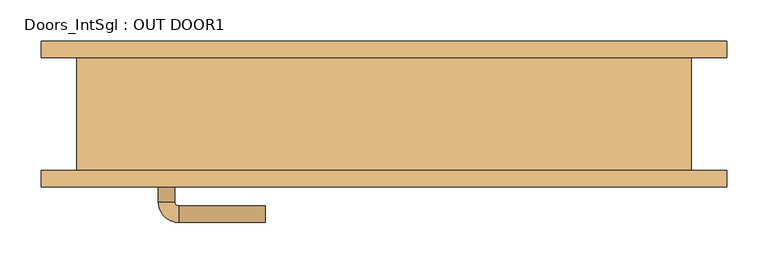
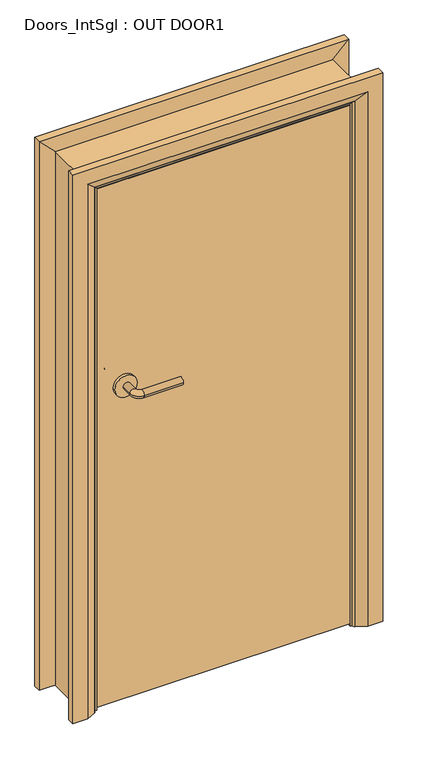
"""IFC4 building model written with IfcOpenShell, lengths in millimetres: door geometry, Doors_IntSgl : OUT DOOR1."""

from ifc_helpers import new_model, si_unit, point, frame, frame_2d, origin, place, context, project, spatial, polyline, circle_curve, ellipse_curve, trimmed, segment, composite_curve, outline, extrude, faceted_brep, source, transform, mapped, element, save
from ifc_brep_helpers import plane_surface, cylinder_surface, revolved_surface, advanced_brep


def doors_intsgl_out_door1_d16f2837(model_context):
    return source(origin(), model_context, "Body", "SolidModel", [
        advanced_brep(
        [(-274.0, -22.58, 900.0), (-254.0, -22.58, 900.0), (-274.0, 7.42, 900.0), (-254.0, 7.42, 900.0), (-249.0, 12.42, 900.0), (-249.0, 32.42, 900.0), (-144.0, 32.42, 900.0), (-144.0, 12.42, 900.0)],
        [
            (0, 1, circle_curve(frame((-264.0, -22.58, 900.0), z_axis=(0.0, -1.0, 0.0), x_axis=(1.0, 0.0, 0.0)), 10.0)),
            (1, 0, circle_curve(frame((-264.0, -22.58, 900.0), z_axis=(0.0, -1.0, 0.0), x_axis=(1.0, 0.0, 0.0)), 10.0)),
            (0, 2),
            (2, 3, circle_curve(frame((-264.0, 7.42, 900.0), z_axis=(0.0, -1.0, 0.0), x_axis=(1.0, 0.0, 0.0)), 10.0)),
            (3, 1),
            (3, 2, circle_curve(frame((-264.0, 7.42, 900.0), z_axis=(0.0, -1.0, 0.0), x_axis=(1.0, 0.0, 0.0)), 10.0)),
            (4, 3, circle_curve(frame((-249.0, 7.42, 900.0), z_axis=(0.0, 0.0, 1.0), x_axis=(-1.0, 0.0, 0.0)), 5.0)),
            (2, 5, circle_curve(frame((-249.0, 7.42, 900.0), z_axis=(0.0, 0.0, -1.0), x_axis=(-1.0, 0.0, 0.0)), 25.0)),
            (5, 4, circle_curve(frame((-249.0, 22.42, 900.0), z_axis=(-1.0, 0.0, 0.0), x_axis=(0.0, -1.0, 0.0)), 10.0)),
            (4, 5, circle_curve(frame((-249.0, 22.42, 900.0), z_axis=(-1.0, 0.0, 0.0), x_axis=(0.0, -1.0, 0.0)), 10.0)),
            (6, 7, circle_curve(frame((-144.0, 22.42, 900.0), z_axis=(1.0, 0.0, 0.0), x_axis=(0.0, -1.0, 0.0)), 10.0)),
            (7, 6, circle_curve(frame((-144.0, 22.42, 900.0), z_axis=(1.0, 0.0, 0.0), x_axis=(0.0, -1.0, 0.0)), 10.0)),
            (5, 6),
            (7, 4),
        ],
        [
            plane_surface(frame((-264.0, -22.58, 900.0), z_axis=(0.0, -1.0, 0.0), x_axis=(0.0, 0.0, 1.0))),
            cylinder_surface(frame((-264.0, -22.58, 900.0), z_axis=(0.0, -1.0, 0.0), x_axis=(1.0, 0.0, 0.0)), 10.0),
            revolved_surface(trimmed(ellipse_curve(frame((-264.0, 7.42, 900.0), z_axis=(0.0, -1.0, 0.0), x_axis=(1.0, 0.0, 0.0)), 10.0, 10.0), [point((-274.0, 7.42, 900.0))], [point((-254.0, 7.42, 900.0))], True, "CARTESIAN"), (-249.0, 7.42, 900.0), (0.0, 0.0, -1.0)),
            revolved_surface(trimmed(ellipse_curve(frame((-264.0, 7.42, 900.0), z_axis=(0.0, -1.0, 0.0), x_axis=(1.0, 0.0, 0.0)), 10.0, 10.0), [point((-254.0, 7.42, 900.0))], [point((-274.0, 7.42, 900.0))], True, "CARTESIAN"), (-249.0, 7.42, 900.0), (0.0, 0.0, -1.0)),
            plane_surface(frame((-144.0, 22.42, 900.0), z_axis=(1.0, 0.0, 0.0), x_axis=(0.0, 0.0, 1.0))),
            cylinder_surface(frame((-249.0, 22.42, 900.0), z_axis=(-1.0, 0.0, 0.0), x_axis=(0.0, -1.0, 0.0)), 10.0),
        ],
        [
            (0, [[1, 2]]),
            (1, [[-1, 3, 4, 5]]),
            (1, [[-2, -5, 6, -3]]),
            (2, [[7, -4, 8, 9]]),
            (3, [[-8, -6, -7, 10]]),
            (4, [[11, 12]]),
            (5, [[-9, 13, -12, 14]]),
            (5, [[-10, -14, -11, -13]]),
        ],
    ),
        extrude(outline(composite_curve([segment(trimmed(circle_curve(frame_2d((900.0, -266.5)), 30.0), [point((900.0, -296.5))], [point((900.0, -236.5))], False, "CARTESIAN"), True, "CONTINUOUS"), segment(trimmed(circle_curve(frame_2d((900.0, -266.5)), 30.0), [point((900.0, -236.5))], [point((900.0, -296.5))], False, "CARTESIAN"), True, "CONTINUOUS")], self_intersect=False)), frame((0.0, -30.58, 0.0), z_axis=(0.0, 1.0, 0.0), x_axis=(0.0, 0.0, 1.0)), (0.0, 0.0, 1.0), 8.0),
        advanced_brep(
        [(-274.0, -76.58, 900.0), (-254.0, -76.58, 900.0), (-254.0, -106.58, 900.0), (-274.0, -106.58, 900.0), (-249.0, -111.58, 900.0), (-249.0, -131.58, 900.0), (-144.0, -131.58, 900.0), (-144.0, -111.58, 900.0)],
        [
            (0, 1, circle_curve(frame((-264.0, -76.58, 900.0), z_axis=(0.0, 1.0, 0.0), x_axis=(1.0, 0.0, 0.0)), 10.0)),
            (1, 0, circle_curve(frame((-264.0, -76.58, 900.0), z_axis=(0.0, 1.0, 0.0), x_axis=(1.0, 0.0, 0.0)), 10.0)),
            (1, 2),
            (2, 3, circle_curve(frame((-264.0, -106.58, 900.0), z_axis=(0.0, 1.0, 0.0), x_axis=(1.0, 0.0, 0.0)), 10.0)),
            (3, 0),
            (3, 2, circle_curve(frame((-264.0, -106.58, 900.0), z_axis=(0.0, 1.0, 0.0), x_axis=(1.0, 0.0, 0.0)), 10.0)),
            (4, 5, circle_curve(frame((-249.0, -121.58, 900.0), z_axis=(-1.0, 0.0, 0.0), x_axis=(0.0, 1.0, 0.0)), 10.0)),
            (5, 3, circle_curve(frame((-249.0, -106.58, 900.0), z_axis=(0.0, 0.0, -1.0), x_axis=(-1.0, 0.0, 0.0)), 25.0)),
            (2, 4, circle_curve(frame((-249.0, -106.58, 900.0), z_axis=(0.0, 0.0, 1.0), x_axis=(-1.0, 0.0, 0.0)), 5.0)),
            (5, 4, circle_curve(frame((-249.0, -121.58, 900.0), z_axis=(-1.0, 0.0, 0.0), x_axis=(0.0, 1.0, 0.0)), 10.0)),
            (6, 7, circle_curve(frame((-144.0, -121.58, 900.0), z_axis=(1.0, 0.0, 0.0), x_axis=(0.0, 1.0, 0.0)), 10.0)),
            (7, 6, circle_curve(frame((-144.0, -121.58, 900.0), z_axis=(1.0, 0.0, 0.0), x_axis=(0.0, 1.0, 0.0)), 10.0)),
            (4, 7),
            (6, 5),
        ],
        [
            plane_surface(frame((-264.0, -76.58, 900.0), z_axis=(0.0, 1.0, 0.0), x_axis=(0.0, 0.0, 1.0))),
            cylinder_surface(frame((-264.0, -76.58, 900.0), z_axis=(0.0, 1.0, 0.0), x_axis=(1.0, 0.0, 0.0)), 10.0),
            revolved_surface(trimmed(ellipse_curve(frame((-264.0, -106.58, 900.0), z_axis=(0.0, -1.0, 0.0), x_axis=(1.0, 0.0, 0.0)), 10.0, 10.0), [point((-274.0, -106.58, 900.0))], [point((-254.0, -106.58, 900.0))], True, "CARTESIAN"), (-249.0, -106.58, 900.0), (0.0, 0.0, -1.0)),
            revolved_surface(trimmed(ellipse_curve(frame((-264.0, -106.58, 900.0), z_axis=(0.0, -1.0, 0.0), x_axis=(1.0, 0.0, 0.0)), 10.0, 10.0), [point((-254.0, -106.58, 900.0))], [point((-274.0, -106.58, 900.0))], True, "CARTESIAN"), (-249.0, -106.58, 900.0), (0.0, 0.0, -1.0)),
            plane_surface(frame((-144.0, -121.58, 900.0), z_axis=(1.0, 0.0, 0.0), x_axis=(0.0, 0.0, 1.0))),
            cylinder_surface(frame((-249.0, -121.58, 900.0), z_axis=(-1.0, 0.0, 0.0), x_axis=(0.0, 1.0, 0.0)), 10.0),
        ],
        [
            (0, [[1, 2]]),
            (1, [[3, 4, 5, -2]]),
            (1, [[-5, 6, -3, -1]]),
            (2, [[7, 8, -4, 9]]),
            (3, [[10, -9, -6, -8]]),
            (4, [[11, 12]]),
            (5, [[13, -11, 14, -7]]),
            (5, [[-14, -12, -13, -10]]),
        ],
    ),
        extrude(outline(composite_curve([segment(trimmed(circle_curve(frame_2d((900.0, -266.5)), 30.0), [point((900.0, -296.5))], [point((900.0, -236.5))], False, "CARTESIAN"), True, "CONTINUOUS"), segment(trimmed(circle_curve(frame_2d((900.0, -266.5)), 30.0), [point((900.0, -236.5))], [point((900.0, -296.5))], False, "CARTESIAN"), True, "CONTINUOUS")], self_intersect=False)), frame((0.0, -76.58, 0.0), z_axis=(0.0, 1.0, 0.0), x_axis=(0.0, 0.0, 1.0)), (0.0, 0.0, 1.0), 8.0),
        extrude(outline(polyline([(339.0, -30.58), (339.0, -68.58), (-339.0, -68.58), (-339.0, -30.58), (339.0, -30.58)])), frame((0.0, 0.0, 8.0), z_axis=(0.0, 0.0, 1.0), x_axis=(1.0, 0.0, 0.0)), (0.0, 0.0, 1.0), 1474.0),
        advanced_brep(
        [(416.0, -88.58, 0.0), (376.0, -88.58, 0.0), (350.0, -74.58, 0.0), (346.0, -68.58, 0.0), (416.0, -68.58, 0.0), (416.0, -68.58, 1559.0), (416.0, -88.58, 1559.0), (346.0, -68.58, 1489.0), (-346.0, -68.58, 1489.0), (-346.0, -68.58, 0.0), (-416.0, -68.58, 0.0), (-416.0, -68.58, 1559.0), (350.0, -74.58, 1493.0), (376.0, -88.58, 1519.0), (-416.0, -88.58, 1559.0), (-416.0, -88.58, 0.0), (-376.0, -88.58, 0.0), (-376.0, -88.58, 1519.0), (-350.0, -74.58, 0.0), (-350.0, -74.58, 1493.0)],
        [
            (0, 1),
            (1, 2),
            (2, 3, circle_curve(frame((354.0, -67.58, 0.0), z_axis=(0.0, 0.0, -1.0), x_axis=(1.0, 0.0, 0.0)), 8.0622577)),
            (3, 4),
            (4, 0),
            (4, 5),
            (5, 6),
            (6, 0),
            (3, 7),
            (7, 8),
            (8, 9),
            (9, 10),
            (10, 11),
            (11, 5),
            (2, 12),
            (12, 7, ellipse_curve(frame((354.0, -67.58, 1497.0), z_axis=(0.7071067811865475, 0.0, -0.7071067811865475), x_axis=(-0.7071067811865474, 0.0, -0.7071067811865476)), 11.4017543, 8.0622577)),
            (1, 13),
            (13, 12),
            (6, 14),
            (14, 15),
            (15, 16),
            (16, 17),
            (17, 13),
            (10, 15),
            (14, 11),
            (9, 18, circle_curve(frame((-354.0, -67.58, 0.0), z_axis=(0.0, 0.0, -1.0), x_axis=(-1.0, 0.0, 0.0)), 8.0622577)),
            (18, 16),
            (19, 18),
            (8, 19, ellipse_curve(frame((-354.0, -67.58, 1497.0), z_axis=(-0.7071067811865475, 0.0, -0.7071067811865475), x_axis=(-0.7071067811865474, 0.0, 0.7071067811865476)), 11.4017543, 8.0622577)),
            (19, 17),
            (12, 19),
        ],
        [
            plane_surface(frame((346.0, -68.58, 0.0), z_axis=(0.0, 0.0, -1.0), x_axis=(0.0, 1.0, 0.0))),
            plane_surface(frame((416.0, -88.58, 0.0), z_axis=(1.0, 0.0, 0.0), x_axis=(0.0, 0.0, 1.0))),
            plane_surface(frame((416.0, -68.58, 0.0), z_axis=(0.0, 1.0, 0.0), x_axis=(0.0, 0.0, 1.0))),
            cylinder_surface(frame((354.0, -67.58, 0.0), z_axis=(0.0, 0.0, -1.0), x_axis=(1.0, 0.0, 0.0)), 8.0622577),
            plane_surface(frame((350.0, -74.58, 0.0), z_axis=(-0.4740998230350126, -0.880471099922178, 0.0), x_axis=(0.0, 0.0, 1.0))),
            plane_surface(frame((376.0, -88.58, 0.0), z_axis=(0.0, -1.0, 0.0), x_axis=(0.0, 0.0, 1.0))),
            plane_surface(frame((-416.0, -88.58, 1559.0), z_axis=(-1.0, 0.0, 0.0), x_axis=(0.0, 0.0, -1.0))),
            plane_surface(frame((-346.0, -68.58, 0.0), z_axis=(0.0, 0.0, -1.0), x_axis=(0.0, 1.0, 0.0))),
            cylinder_surface(frame((-354.0, -67.58, 1489.0), z_axis=(0.0, 0.0, 1.0), x_axis=(-1.0, 0.0, 0.0)), 8.0622577),
            plane_surface(frame((-350.0, -74.58, 1493.0), z_axis=(0.47409982303501824, -0.8804710999221749, 0.0), x_axis=(0.0, 0.0, -1.0))),
            plane_surface(frame((416.0, -88.58, 1559.0), z_axis=(0.0, 0.0, 1.0), x_axis=(-1.0, 0.0, 0.0))),
            cylinder_surface(frame((346.0, -67.58, 1497.0), z_axis=(1.0, 0.0, 0.0), x_axis=(0.0, 0.0, 1.0)), 8.0622577),
            plane_surface(frame((350.0, -74.58, 1493.0), z_axis=(0.0, -0.8804710999221764, -0.4740998230350154), x_axis=(-1.0, 0.0, 0.0))),
        ],
        [
            (0, [[1, 2, 3, 4, 5]]),
            (1, [[6, 7, 8, -5]]),
            (2, [[9, 10, 11, 12, 13, 14, -6, -4]]),
            (3, [[15, 16, -9, -3]]),
            (4, [[17, 18, -15, -2]]),
            (5, [[-8, 19, 20, 21, 22, 23, -17, -1]]),
            (6, [[-13, 24, -20, 25]]),
            (7, [[-24, -12, 26, 27, -21]]),
            (8, [[28, -26, -11, 29]]),
            (9, [[-22, -27, -28, 30]]),
            (10, [[-14, -25, -19, -7]]),
            (11, [[31, -29, -10, -16]]),
            (12, [[-23, -30, -31, -18]]),
        ],
    ),
        advanced_brep(
        [(-416.0, 88.58, 0.0), (-376.0, 88.58, 0.0), (-350.0, 74.58, 0.0), (-346.0, 68.58, 0.0), (-416.0, 68.58, 0.0), (-416.0, 68.58, 1559.0), (-416.0, 88.58, 1559.0), (-346.0, 68.58, 1489.0), (-350.0, 74.58, 1493.0), (-376.0, 88.58, 1519.0), (416.0, 88.58, 0.0), (416.0, 68.58, 0.0), (346.0, 68.58, 0.0), (350.0, 74.58, 0.0), (376.0, 88.58, 0.0), (416.0, 88.58, 1559.0), (376.0, 88.58, 1519.0), (350.0, 74.58, 1493.0), (346.0, 68.58, 1489.0), (416.0, 68.58, 1559.0)],
        [
            (0, 1),
            (1, 2),
            (2, 3, circle_curve(frame((-354.0, 67.58, 0.0), z_axis=(0.0, 0.0, -1.0), x_axis=(-1.0, 0.0, 0.0)), 8.0622577)),
            (3, 4),
            (4, 0),
            (4, 5),
            (5, 6),
            (6, 0),
            (3, 7),
            (7, 5),
            (2, 8),
            (8, 7, ellipse_curve(frame((-354.0, 67.58, 1497.0), z_axis=(-0.7071067811865475, 0.0, -0.7071067811865475), x_axis=(0.7071067811865474, 0.0, -0.7071067811865476)), 11.4017543, 8.0622577)),
            (1, 9),
            (9, 8),
            (6, 9),
            (10, 11),
            (11, 12),
            (12, 13, circle_curve(frame((354.0, 67.58, 0.0), z_axis=(0.0, 0.0, -1.0), x_axis=(1.0, 0.0, 0.0)), 8.0622577)),
            (13, 14),
            (14, 10),
            (15, 10),
            (14, 16),
            (16, 15),
            (13, 17),
            (17, 16),
            (12, 18),
            (18, 17, ellipse_curve(frame((354.0, 67.58, 1497.0), z_axis=(0.7071067811865475, 0.0, -0.7071067811865475), x_axis=(0.7071067811865474, 0.0, 0.7071067811865476)), 11.4017543, 8.0622577)),
            (11, 19),
            (19, 18),
            (15, 19),
            (5, 19),
            (15, 6),
            (7, 18),
            (8, 17),
            (9, 16),
        ],
        [
            plane_surface(frame((-346.0, 141.3810989, 0.0), z_axis=(0.0, 0.0, -1.0), x_axis=(1.0, 0.0, 0.0))),
            plane_surface(frame((-416.0, 88.58, 0.0), z_axis=(-1.0, 0.0, 0.0), x_axis=(0.0, 0.0, 1.0))),
            plane_surface(frame((-416.0, 68.58, 0.0), z_axis=(0.0, -1.0, 0.0), x_axis=(0.0, 0.0, 1.0))),
            cylinder_surface(frame((-354.0, 67.58, 0.0), z_axis=(0.0, 0.0, -1.0), x_axis=(-1.0, 0.0, 0.0)), 8.0622577),
            plane_surface(frame((-350.0, 74.58, 0.0), z_axis=(0.4740998230350183, 0.8804710999221749, 0.0), x_axis=(0.0, 0.0, 1.0))),
            plane_surface(frame((-376.0, 88.58, 0.0), z_axis=(0.0, 1.0, 0.0), x_axis=(0.0, 0.0, 1.0))),
            plane_surface(frame((346.0, 141.3810989, 0.0), z_axis=(0.0, 0.0, -1.0), x_axis=(-1.0, 0.0, 0.0))),
            plane_surface(frame((376.0, 88.58, 1519.0), z_axis=(0.0, 1.0, 0.0), x_axis=(0.0, 0.0, -1.0))),
            plane_surface(frame((350.0, 74.58, 1493.0), z_axis=(-0.4740998230350183, 0.8804710999221749, 0.0), x_axis=(0.0, 0.0, -1.0))),
            cylinder_surface(frame((354.0, 67.58, 1489.0), z_axis=(0.0, 0.0, 1.0), x_axis=(1.0, 0.0, 0.0)), 8.0622577),
            plane_surface(frame((416.0, 68.58, 1559.0), z_axis=(0.0, -1.0, 0.0), x_axis=(0.0, 0.0, -1.0))),
            plane_surface(frame((416.0, 88.58, 1559.0), z_axis=(1.0, 0.0, 0.0), x_axis=(0.0, 0.0, -1.0))),
            plane_surface(frame((-416.0, 88.58, 1559.0), z_axis=(0.0, 0.0, 1.0), x_axis=(1.0, 0.0, 0.0))),
            plane_surface(frame((-416.0, 68.58, 1559.0), z_axis=(0.0, -1.0, 0.0), x_axis=(1.0, 0.0, 0.0))),
            cylinder_surface(frame((-346.0, 67.58, 1497.0), z_axis=(-1.0, 0.0, 0.0), x_axis=(0.0, 0.0, 1.0)), 8.0622577),
            plane_surface(frame((-350.0, 74.58, 1493.0), z_axis=(0.0, 0.8804710999221749, -0.4740998230350183), x_axis=(1.0, 0.0, 0.0))),
            plane_surface(frame((-376.0, 88.58, 1519.0), z_axis=(0.0, 1.0, 0.0), x_axis=(1.0, 0.0, 0.0))),
        ],
        [
            (0, [[1, 2, 3, 4, 5]]),
            (1, [[6, 7, 8, -5]]),
            (2, [[9, 10, -6, -4]]),
            (3, [[11, 12, -9, -3]]),
            (4, [[13, 14, -11, -2]]),
            (5, [[-8, 15, -13, -1]]),
            (6, [[16, 17, 18, 19, 20]]),
            (7, [[21, -20, 22, 23]]),
            (8, [[-22, -19, 24, 25]]),
            (9, [[-24, -18, 26, 27]]),
            (10, [[-26, -17, 28, 29]]),
            (11, [[-28, -16, -21, 30]]),
            (12, [[31, -30, 32, -7]]),
            (13, [[33, -29, -31, -10]]),
            (14, [[34, -27, -33, -12]]),
            (15, [[35, -25, -34, -14]]),
            (16, [[-32, -23, -35, -15]]),
        ],
    ),
        faceted_brep([(-341.0, -68.58, 0.0), (-373.0, -68.58, 0.0), (-373.0, 68.58, 0.0), (-341.0, 68.58, 0.0), (-341.0, 68.58, 1484.0), (-341.0, -68.58, 1484.0), (-373.0, 68.58, 1516.0), (-373.0, -68.58, 1516.0), (341.0, -68.58, 0.0), (341.0, 68.58, 0.0), (373.0, 68.58, 0.0), (373.0, -68.58, 0.0), (341.0, -68.58, 1484.0), (373.0, -68.58, 1516.0), (373.0, 68.58, 1516.0), (341.0, 68.58, 1484.0)], [[[0, 1, 2, 3]], [[3, 4, 5, 0]], [[2, 6, 4, 3]], [[1, 7, 6, 2]], [[0, 5, 7, 1]], [[8, 9, 10, 11]], [[12, 8, 11, 13]], [[13, 11, 10, 14]], [[14, 10, 9, 15]], [[15, 9, 8, 12]], [[4, 15, 12, 5]], [[6, 14, 15, 4]], [[7, 13, 14, 6]], [[5, 12, 13, 7]]]),
        extrude(outline(polyline([(0.0, -322.0), (1465.0, -322.0), (1465.0, 322.0), (0.0, 322.0), (0.0, 341.0), (1484.0, 341.0), (1484.0, -341.0), (0.0, -341.0), (0.0, -322.0)])), frame((0.0, -28.58, 0.0), z_axis=(0.0, 1.0, 0.0), x_axis=(0.0, 0.0, 1.0)), (0.0, 0.0, 1.0), 32.0),
    ])


if __name__ == "__main__":
    model = new_model("IFC4")
    model_context = context("Model", 3, world=origin())
    ifc_project = project(units=[si_unit("LENGTHUNIT", "METRE", prefix="MILLI")], contexts=[model_context])
    site = spatial("IfcSite", under=ifc_project)
    building = spatial("IfcBuilding", under=site)
    placement = place(None, origin())
    doors_intsgl_out_door1_shape = doors_intsgl_out_door1_d16f2837(model_context)
    element("IfcDoor", 1, ObjectType="Doors_IntSgl : OUT DOOR1", at=placement, inside=building, context=model_context, shape_type="MappedRepresentation", body=[
        mapped(doors_intsgl_out_door1_shape, transform((0.0, 0.0, 0.0), x_axis=(1.0, 0.0, 0.0), y_axis=(0.0, 1.0, 0.0), z_axis=(0.0, 0.0, 1.0))),
    ])
    save(model, "model.ifc")

# Revit data of these elements
# Type "Doors_IntSgl : OUT DOOR1"
#   Type Mark = "53"
#   Type Comments = "Internal Single"
#   Operation = "SingleSwingRight"
#   Manufacturer = "Revit"
#   Keynote = "L20"
#   Description = "Internal Single Door"
#   Analytic Construction = "Metal"
#   UnderCut = 8 mm
#   Tolerance = 2 mm
#   Thickness = 38 mm
#   Thermal Resistance (R) = 0.270117 (m²·K)/W
#   Structural Tolerance = 8 mm
#   StopDepth = 32 mm
#   Stop Thickness = 19 mm
#   Rough Width = 762 mm
#   Rough Height = 1524 mm
#   Height to Top Lock Rail = 1000 mm
#   Heat Transfer Coefficient (U) = 3.7021 W/(m²·K)
#   Handle Z Distance = 900 mm
#   Handle X Distance = 75 mm
#   Frame Thickness = 32 mm
#   Door Panel Width = 678 mm
#   Door Panel Thickness = 38 mm
#   Door Panel Offset = 0 mm
#   Height = 1524 mm
#   Width = 762 mm
#   Door Panel Height = 1474 mm
#   Architrave Setback = 5 mm
#   Vis - Ironmongery = yes
#   Material Ironmongery = Door - Handle
#   Material Frame = Door - Frame/Mullion (1)
#   Material Door = Door - Panel
#   Material Architrave = Door - Architrave
#   Visual Light Transmittance = 0
#   Solar Heat Gain Coefficient = 0
#   Function = (empty or 0)
#   Wall Closure = (empty or 0)
# Element 1 (IfcDoor, "Doors_IntSgl : OUT DOOR1")
#   Materials on its faces: "Door - Architrave", "Door - Handle", "Door - Frame/Mullion (1)", "Door - Panel"
# Materials
#   "Door - Handle": colour RGB 0 0 0, transparency 0, Keynote = "P21", Cost = 0
#   "Door - Frame/Mullion (1)": class "Wood", colour RGB 212 179 113, transparency 0, Keynote = "L20", Cost = 0
#   "Door - Panel": class "Wood", colour RGB 210 159 95, transparency 0, Keynote = "L20", Cost = 0
#   "Door - Architrave": class "Wood", colour RGB 154 90 5, transparency 0, Keynote = "P20", Cost = 0
